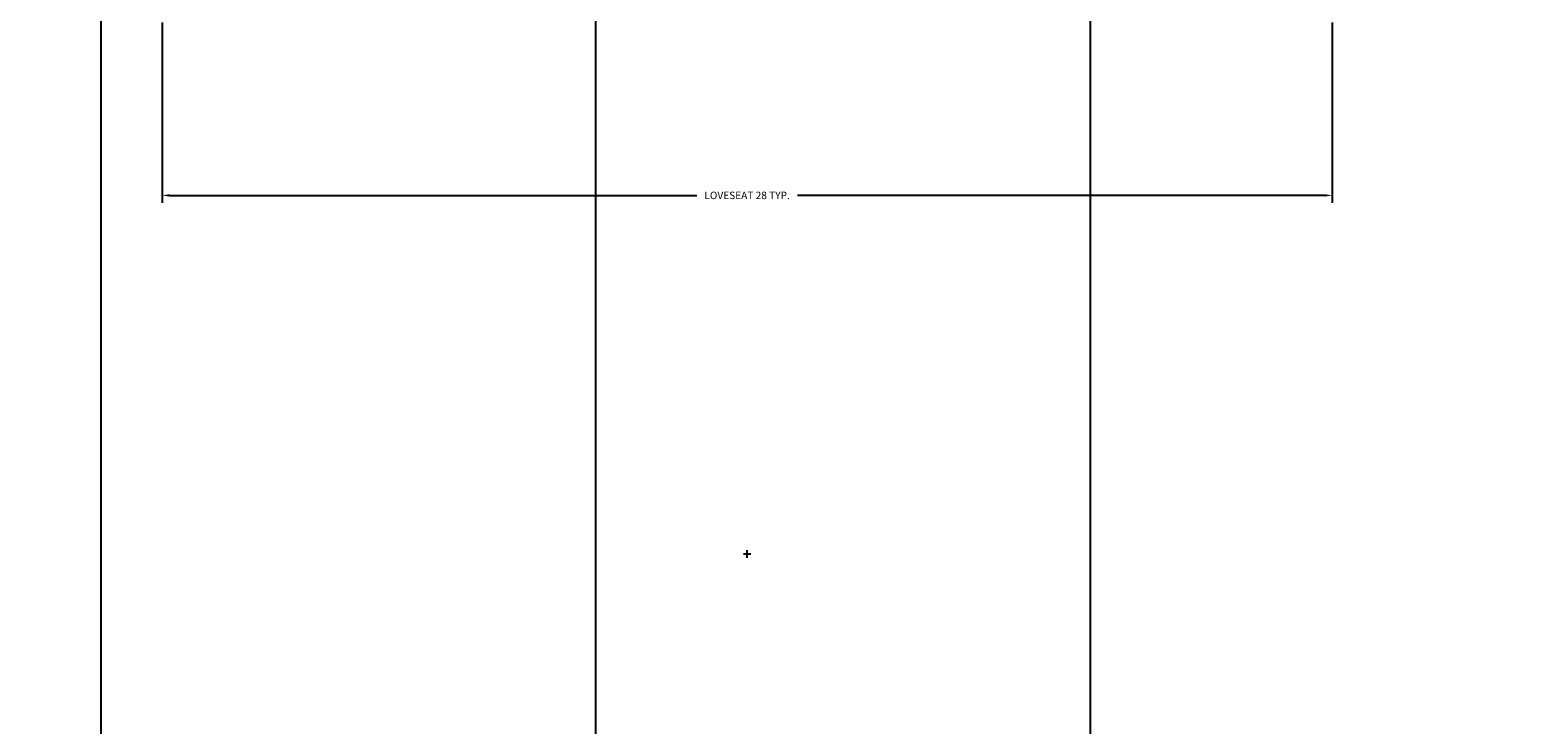
# Model space of a CAD drawing. Units: feet. Extents: x 1654 to 2985, y 1348 to 2230.
# Tile 48 of 53: x 2723 to 2759, y 1842 to 1859. Entities that reach past the tile are written whole.
import ezdxf

# ---------------------------------------------------------------- set-up
doc = ezdxf.new("R2010")
doc.units = ezdxf.units.FT
doc.layers.add('A-ANNO-DIMS', color=2, linetype='Continuous', lineweight=18)
doc.styles.get("Standard").update_dxf_attribs({"font": 'arial.ttf'})
doc.dimstyles.get("Standard").update_dxf_attribs({"dimtxt": 0.18, "dimasz": 0.18, "dimexe": 0.18, "dimexo": 0.0625, "dimgap": 0.09, "dimtad": 0, "dimtih": 1, "dimtoh": 1, "dimdec": 4, "dimzin": 0, "dimdsep": 46, "dimtxsty": 'Standard', "dimcen": 0.09, "dimadec": 0, "dimazin": 0, "dimtfac": 1, "dimtdec": 4, "dimtofl": 0, "dimtmove": 0, "dimatfit": 3, "dimfxl": 1, "dimtolj": 1, "dimtzin": 0, "dimarcsym": 0})

# ---------------------------------------------------------------- blocks, each defined once
blk = doc.blocks.new('*D40')
at = {"layer": 'A-ANNO-DIMS', "color": 0, "lineweight": -2, "transparency": 16777216}
for p, q in [((2726.19, 1859.009), (2726.19, 1854.635)), ((2754.563, 1859.009), (2754.563, 1854.635)), ((2726.37, 1854.815), (2739.154, 1854.815)), ((2754.383, 1854.815), (2741.599, 1854.815))]:
    blk.add_line(p, q, dxfattribs=at)
at = {"layer": 'A-ANNO-DIMS', "color": 0, "transparency": 16777216}
for points in [[(2726.37, 1854.845), (2726.37, 1854.785), (2726.19, 1854.815)], [(2754.383, 1854.845), (2754.383, 1854.785), (2754.563, 1854.815)]]:
    blk.add_solid(points, dxfattribs=at)
at = {"layer": 'Defpoints', "color": 0, "transparency": 16777216}
for p in [(2726.19, 1859.071), (2754.563, 1859.071), (2754.563, 1854.815)]:
    blk.add_point(p, dxfattribs=at)
at = {"layer": 'A-ANNO-DIMS', "color": 0, "transparency": 16777216, "insert": (2740.376, 1854.815), "char_height": 0.18, "attachment_point": 5}
blk.add_mtext('\\A1;LOVESEAT 28 TYP.', dxfattribs=at)
blk = doc.blocks.new('*D82')
at = {"layer": 'A-ANNO-DIMS', "color": 0, "lineweight": -2, "transparency": 16777216}
for p, q in [((2652.706, 2039.192), (2652.706, 1490.625)), ((2784.706, 2039.192), (2784.706, 1490.625)), ((2652.886, 1490.805), (2718.426, 1490.805)), ((2784.526, 1490.805), (2718.985, 1490.805))]:
    blk.add_line(p, q, dxfattribs=at)
at = {"layer": 'A-ANNO-DIMS', "color": 0, "transparency": 16777216}
for points in [[(2652.886, 1490.835), (2652.886, 1490.775), (2652.706, 1490.805)], [(2784.526, 1490.835), (2784.526, 1490.775), (2784.706, 1490.805)]]:
    blk.add_solid(points, dxfattribs=at)
at = {"layer": 'Defpoints', "color": 0, "transparency": 16777216}
for p in [(2652.706, 2039.255), (2784.706, 2039.255), (2784.706, 1490.805)]:
    blk.add_point(p, dxfattribs=at)
at = {"layer": 'A-ANNO-DIMS', "color": 0, "transparency": 16777216, "insert": (2718.706, 1490.805), "char_height": 0.18, "attachment_point": 5}
blk.add_mtext('\\A1;132', dxfattribs=at)
blk = doc.blocks.new('*D86')
at = {"layer": 'A-ANNO-DIMS', "color": 0, "lineweight": -2, "transparency": 16777216}
for p, q in [((2748.706, 1616.317), (2748.706, 2149.885)), ((2784.706, 1607.317), (2784.706, 2149.885)), ((2748.886, 2149.705), (2766.487, 2149.705)), ((2784.526, 2149.705), (2766.925, 2149.705))]:
    blk.add_line(p, q, dxfattribs=at)
at = {"layer": 'A-ANNO-DIMS', "color": 0, "transparency": 16777216}
for points in [[(2748.886, 2149.735), (2748.886, 2149.675), (2748.706, 2149.705)], [(2784.526, 2149.735), (2784.526, 2149.675), (2784.706, 2149.705)]]:
    blk.add_solid(points, dxfattribs=at)
at = {"layer": 'Defpoints', "color": 0, "transparency": 16777216}
for p in [(2784.706, 2149.705), (2748.706, 1616.255), (2784.706, 1607.255)]:
    blk.add_point(p, dxfattribs=at)
at = {"layer": 'A-ANNO-DIMS', "color": 0, "transparency": 16777216, "insert": (2766.706, 2149.705), "char_height": 0.18, "attachment_point": 5}
blk.add_mtext('\\A1;36', dxfattribs=at)
blk = doc.blocks.new('*D87')
at = {"layer": 'A-ANNO-DIMS', "color": 0, "lineweight": -2, "transparency": 16777216}
for p, q in [((2724.706, 1565.317), (2724.706, 2149.885)), ((2736.706, 1565.317), (2736.706, 2149.885)), ((2724.886, 2149.705), (2730.496, 2149.705)), ((2736.526, 2149.705), (2730.915, 2149.705))]:
    blk.add_line(p, q, dxfattribs=at)
at = {"layer": 'A-ANNO-DIMS', "color": 0, "transparency": 16777216}
for points in [[(2724.886, 2149.735), (2724.886, 2149.675), (2724.706, 2149.705)], [(2736.526, 2149.735), (2736.526, 2149.675), (2736.706, 2149.705)]]:
    blk.add_solid(points, dxfattribs=at)
at = {"layer": 'Defpoints', "color": 0, "transparency": 16777216}
for p in [(2736.706, 2149.705), (2724.706, 1565.255), (2736.706, 1565.255)]:
    blk.add_point(p, dxfattribs=at)
at = {"layer": 'A-ANNO-DIMS', "color": 0, "transparency": 16777216, "insert": (2730.706, 2149.705), "char_height": 0.18, "attachment_point": 5}
blk.add_mtext('\\A1;12', dxfattribs=at)
blk = doc.blocks.new('*D111')
at = {"layer": 'A-ANNO-DIMS', "color": 0, "lineweight": -2, "transparency": 16777216}
for p, q in [((2740.196, 1888.027), (2740.376, 1888.027)), ((2740.376, 1888.027), (2740.376, 1872.492)), ((2740.286, 1846.122), (2740.466, 1846.122)), ((2740.376, 1846.032), (2740.376, 1846.212))]:
    blk.add_line(p, q, dxfattribs=at)
at = {"layer": 'A-ANNO-DIMS', "color": 0, "transparency": 16777216}
blk.add_solid([(2740.406, 1872.492), (2740.346, 1872.492), (2740.376, 1872.312)], dxfattribs=at)
at = {"layer": 'Defpoints', "color": 0, "transparency": 16777216}
for p in [(2740.376, 1872.312), (2740.376, 1846.122)]:
    blk.add_point(p, dxfattribs=at)
at = {"layer": 'A-ANNO-DIMS', "color": 0, "transparency": 16777216, "insert": (2739.521, 1888.027), "char_height": 0.18, "attachment_point": 5}
blk.add_mtext('\\A1;2X R26.19', dxfattribs=at)

msp = doc.modelspace()

# ---------------------------------------------------------------- dimensions: what is measured, and where the dimension line sits
at = {"layer": 'A-ANNO-DIMS'}
for base, p1, p2, picture, middle in [((2736.7058, 2149.7049), (2724.7058, 1565.2549), (2736.7058, 1565.2549), '*D87', (2730.7058, 2149.7049)), ((2784.7058, 2149.7049), (2748.7058, 1616.2549), (2784.7058, 1607.2549), '*D86', (2766.7058, 2149.7049)), ((2784.7058, 1490.8049), (2652.7058, 2039.2549), (2784.7058, 2039.2549), '*D82', (2718.7058, 1490.8049))]:
    dim = msp.add_linear_dim(base=base, p1=p1, p2=p2, dimstyle='Standard', override={"dimdec": 0, "dimlfac": 1, "dimrnd": 0, "dimzin": 0, "dimdsep": 46, "dimlunit": 2}, dxfattribs=at)
    dim.commit()
    dim.dimension.update_dxf_attribs({"geometry": picture, "text_midpoint": middle})
dim = msp.add_radius_dim(center=(2740.3765, 1846.1218), mpoint=(2740.376, 1872.3123), text='2X <>', dimstyle='Standard', override={"dimdec": 2, "dimlfac": 1, "dimrnd": 0, "dimzin": 0, "dimdsep": 46, "dimlunit": 2}, dxfattribs=at)
dim.commit()
dim.dimension.update_dxf_attribs({"geometry": '*D111', "text_midpoint": (2739.5208, 1888.0267), "dimtype": 164})
dim = msp.add_linear_dim(base=(2754.5631, 1854.8155), p1=(2726.1899, 1859.0715), p2=(2754.5631, 1859.0715), text='LOVESEAT <> TYP.', dimstyle='Standard', override={"dimdec": 0, "dimlfac": 1, "dimrnd": 0, "dimzin": 0, "dimdsep": 46, "dimlunit": 2}, dxfattribs=at)
dim.commit()
dim.dimension.update_dxf_attribs({"geometry": '*D40', "text_midpoint": (2740.3765, 1854.8155)})

doc.saveas('drawing.dxf')
